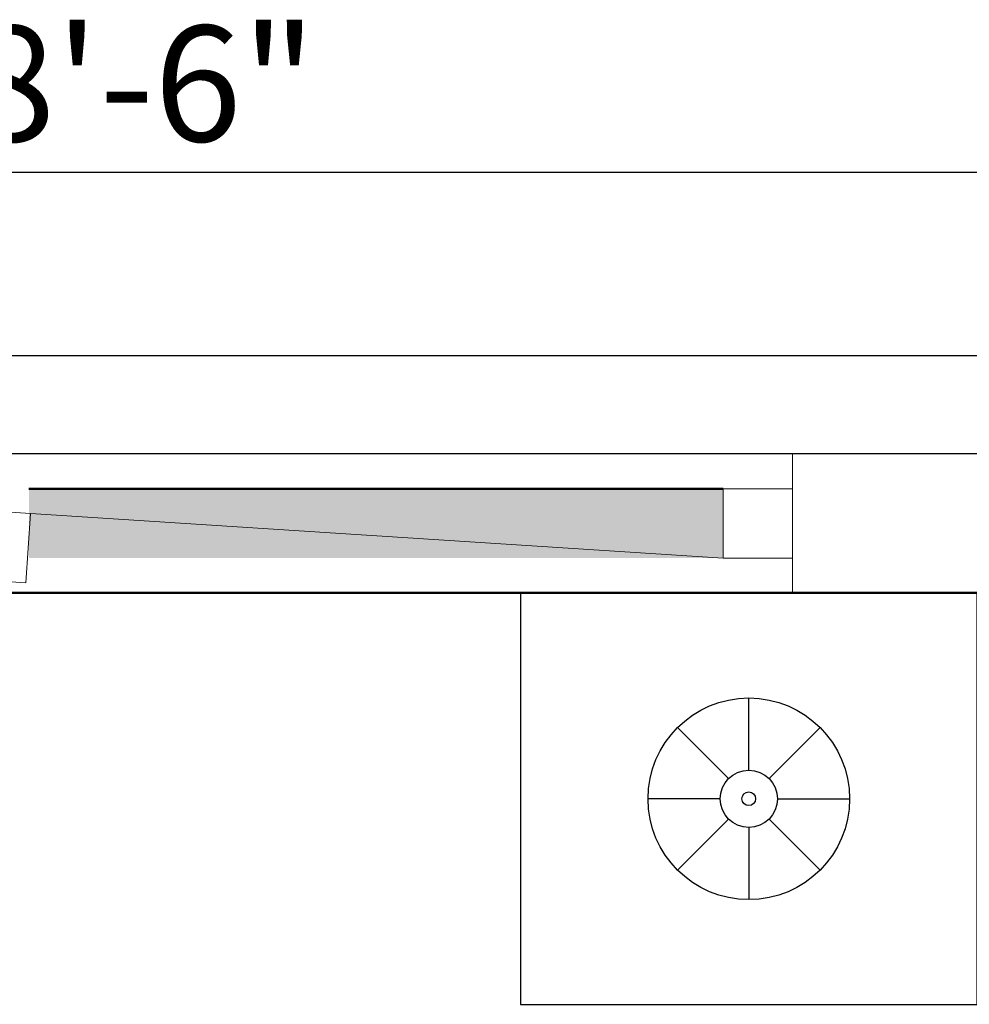
# Model space of a CAD drawing. Units: inches. Extents: x 3064 to 19385, y 846 to 15425.
# Tile 30 of 108: x 4932 to 4973, y 1368 to 1411. Entities that reach past the tile are written whole.
import ezdxf

# ---------------------------------------------------------------- set-up
doc = ezdxf.new("R2010")
doc.units = ezdxf.units.IN
for name, color, linetype, lineweight in [('A-ANNO-DIMS', 2, 'Continuous', 18), ('A-FLOR-FIXT', 9, 'Continuous', 18), ('A-GLAZ', 4, 'Continuous', 18), ('A-WALL', 7, 'Continuous', 50), ('C-PROP', 6, 'Continuous', 25)]:
    doc.layers.add(name, color=color, linetype=linetype, lineweight=lineweight)
doc.layers.add('BLOCK', color=6, linetype='Continuous')
doc.styles.get("Standard").update_dxf_attribs({"font": 'arial.ttf'})
doc.dimstyles.new('ISO-25', dxfattribs={"dimtxt": 9, "dimasz": 2.5, "dimexe": 1.25, "dimexo": 0.625, "dimtad": 1, "dimdec": 1, "dimlunit": 3, "dimtxsty": 'Standard', "dimcen": 2.5, "dimadec": 0, "dimazin": 0, "dimtfac": 1, "dimtdec": 1, "dimtmove": 0, "dimatfit": 3, "dimfxl": 1, "dimarcsym": 0})

# ---------------------------------------------------------------- blocks, each defined once
blk = doc.blocks.new('A$C52E67D0D')
at = {"layer": 'BLOCK'}
for p, q in [((250.5, 1605.5), (250.5, 1684.7)), ((228.3, 1596.3), (172.3, 1652.3)), ((272.7, 1596.3), (328.7, 1652.3)), ((219.1, 1574.1), (139.9, 1574.1)), ((281.9, 1574.1), (361.1, 1574.1)), ((228.3, 1551.9), (172.3, 1495.9)), ((272.7, 1551.9), (328.7, 1495.9)), ((250.5, 1542.8), (250.5, 1463.5))]:
    blk.add_line(p, q, dxfattribs=at)
blk.add_lwpolyline([(501, 1348.6), (501, 1799.6), (0, 1799.6), (0, 1348.6)], close=True, dxfattribs=at)
for radius in [110.6, 31.4, 7.46]:
    blk.add_circle((250.5, 1574.1), radius, dxfattribs=at)
blk = doc.blocks.new('*D46')
at = {"layer": 'A-ANNO-DIMS', "color": 0, "lineweight": -2, "transparency": 16777216}
for p, q in [((4905.476, 1392.721), (4905.476, 1397.601)), ((5100.476, 1392.721), (5100.476, 1397.601)), ((4907.976, 1396.351), (5097.976, 1396.351))]:
    blk.add_line(p, q, dxfattribs=at)
at = {"layer": 'A-ANNO-DIMS', "color": 0, "transparency": 16777216}
for points in [[(4907.976, 1396.768), (4907.976, 1395.934), (4905.476, 1396.351)], [(5097.976, 1396.768), (5097.976, 1395.934), (5100.476, 1396.351)]]:
    blk.add_solid(points, dxfattribs=at)
at = {"layer": 'Defpoints', "color": 0, "transparency": 16777216}
for p in [(5100.476, 1396.351), (4905.476, 1392.096), (5100.476, 1392.096)]:
    blk.add_point(p, dxfattribs=at)
at = {"layer": 'A-ANNO-DIMS', "color": 0, "transparency": 16777216, "insert": (5002.976, 1399.53), "char_height": 5, "attachment_point": 5}
blk.add_mtext('16\'-3"', dxfattribs=at)
blk = doc.blocks.new('*D67')
at = {"layer": 'A-ANNO-DIMS', "color": 0, "lineweight": -2, "transparency": 16777216}
for p, q in [((4764.476, 1392.721), (4764.476, 1405.519)), ((5106.476, 1392.721), (5106.476, 1405.519)), ((4766.976, 1404.269), (5103.976, 1404.269))]:
    blk.add_line(p, q, dxfattribs=at)
at = {"layer": 'A-ANNO-DIMS', "color": 0, "transparency": 16777216}
for points in [[(4766.976, 1404.686), (4766.976, 1403.852), (4764.476, 1404.269)], [(5103.976, 1404.686), (5103.976, 1403.852), (5106.476, 1404.269)]]:
    blk.add_solid(points, dxfattribs=at)
at = {"layer": 'Defpoints', "color": 0, "transparency": 16777216}
for p in [(5106.476, 1404.269), (4764.476, 1392.096), (5106.476, 1392.096)]:
    blk.add_point(p, dxfattribs=at)
at = {"layer": 'A-ANNO-DIMS', "color": 0, "transparency": 16777216, "insert": (4935.476, 1407.447), "char_height": 5, "attachment_point": 5}
blk.add_mtext('28\'-6"', dxfattribs=at)
blk = doc.blocks.new('WIN-900')
blk.add_line((0, 0), (30, 0))
blk.add_lwpolyline([(30, 0), (30, 3), (33, 3), (33, 0)], close=True)

msp = doc.modelspace()

# ---------------------------------------------------------------- hatches: boundary and pattern name
at = {"layer": 'A-GLAZ'}
h = msp.add_hatch(color=256, dxfattribs=at)
h.dxf.hatch_style = 1
h.paths.add_polyline_path([(4962.476, 1390.596), (4932.476, 1390.596), (4932.476, 1387.596), (4962.476, 1387.596)])

# ---------------------------------------------------------------- linework, layer by layer
msp.add_line((4965.476, 1392.096), (4965.476, 1386.096), dxfattribs=at)
msp.add_lwpolyline([(4965.476, 1387.596), (4962.476, 1387.596), (4962.476, 1390.596), (4965.476, 1390.596)], close=True, dxfattribs=at)
at = {"layer": 'A-WALL'}
for p, q in [((4932.476, 1390.596), (4962.476, 1390.596)), ((5100.476, 1386.096), (4905.476, 1386.096))]:
    msp.add_line(p, q, dxfattribs=at)
at = {"layer": 'C-PROP'}
msp.add_line((5106.476, 1392.096), (4764.476, 1392.096), dxfattribs=at)

# ---------------------------------------------------------------- block references
at = {"layer": 'A-FLOR-FIXT', "xscale": 0.039370099999992, "yscale": 0.039370099999992, "zscale": 0.039370099999992}
msp.add_blockref('A$C52E67D0D', (4953.724, 1315.23), dxfattribs=at)
at = {"layer": 'A-GLAZ', "rotation": 176.3047794680105}
msp.add_blockref('WIN-900', (4962.477, 1387.596), dxfattribs=at)

# ---------------------------------------------------------------- dimensions: what is measured, and where the dimension line sits
at = {"layer": 'A-ANNO-DIMS'}
for base, p1, p2, override, picture, middle in [((5106.476, 1404.269), (4764.476, 1392.096), (5106.476, 1392.096), {"dimtxt": 5, "dimclrd": 0, "dimclre": 0, "dimclrt": 0}, '*D67', (4935.476, 1407.447)), ((5100.476, 1396.351), (4905.476, 1392.096), (5100.476, 1392.096), {"dimtxt": 5, "dimclrd": 0, "dimclre": 0, "dimclrt": 0, "dimtmove": 1}, '*D46', (5002.976, 1399.53))]:
    dim = msp.add_linear_dim(base=base, p1=p1, p2=p2, dimstyle='ISO-25', override=override, dxfattribs=at)
    dim.commit()
    dim.dimension.update_dxf_attribs({"geometry": picture, "text_midpoint": middle})

doc.saveas('drawing.dxf')
